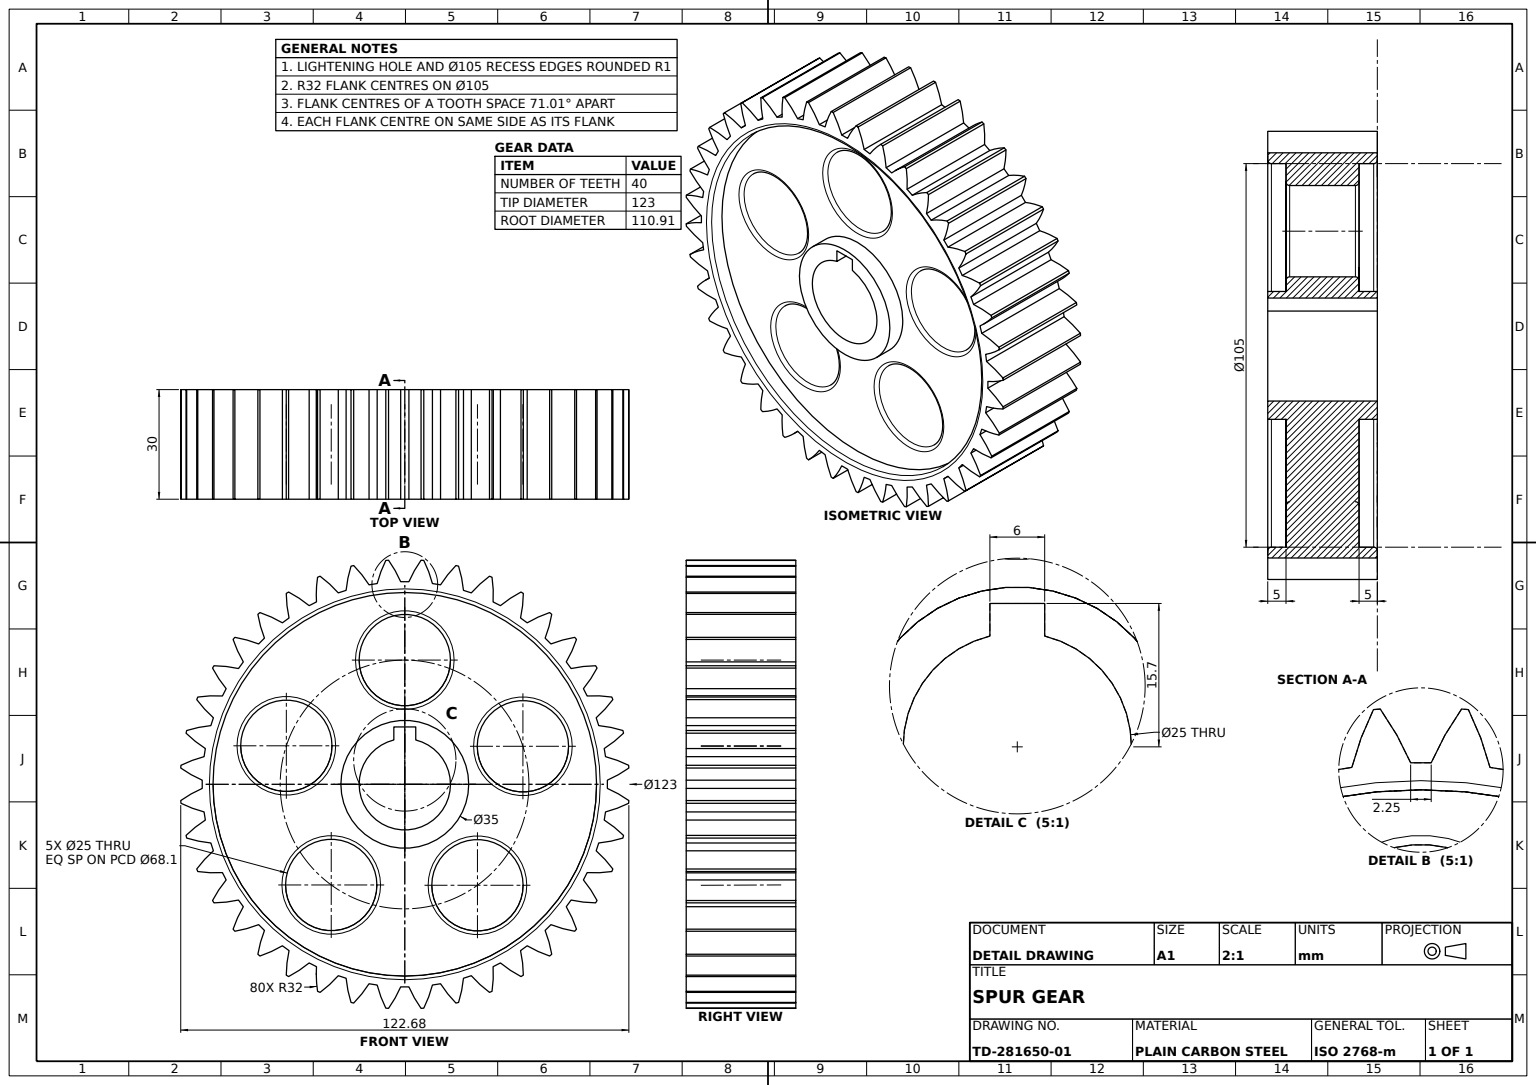
SolidWorks part; units mm, degrees
material "Plain Carbon Steel"
ref_plane "Front Plane" through (0, 0, 0) normal (0, 0, 1) x (1, 0, 0)
ref_plane "Top Plane" through (0, 0, 0) normal (0, 1, 0) x (1, 0, 0)
ref_plane "Right Plane" through (0, 0, 0) normal (1, 0, 0) x (0, 0, -1)
sketch "Gear Blank Sketch" plane through (0, 0, 0) normal (0, 0, 1) x (1, 0, 0)
  line L0 (-71.0252, 0) -> (67.6964, 0) construction
  line L1 (0, 44.8674) -> (0, -38.0607) construction
  line L2 (-3, 12.1347) -> (-3, 15.7)
  line L3 (3, 12.1347) -> (3, 15.7)
  line L4 (-3, 15.7) -> (3, 15.7)
  arc A0 (-3, 12.1347) -> (3, 12.1347) centre (0, 0) ccw
  circle A1 centre (0, 0) radius 61.5
  dimension "D1" = 25
  dimension "D4" = 123
  dimension "D2" = 6
  dimension "D3" = 15.7
extrude "Gear Blank" add sketch "Gear Blank Sketch" along normal blind 30
sketch "Face Recess Sketch" plane through (0, 0, 30) normal (0, 0, 1) x (1, 0, 0)
  circle A0 centre (0, 0) radius 52.5
  dimension "D1" = 105
extrude "Face Recess Ø105" cut sketch "Face Recess Sketch" against normal blind 5
ref_plane "Gear Mid Plane" through (0, 0, 15) normal (0, 0, 1) x (1, 0, 0)
mirror "Face Recess Mirror" about plane through (0, 0, 15) normal (0, 0, 1) of "Face Recess Ø105"
sketch "Tooth Space Sketch" plane through (0, 0, 25) normal (0, 0, 1) x (1, 0, 0)
  line L1 (0, 82.4606) -> (0, -88.1983) construction
  line L2 (-105.0435, 0) -> (137.9983, 0) construction
  line L3 (-1.125, 55.4564) -> (1.125, 55.4564)
  circle A3 centre (0, 0) radius 52.5 construction
  arc A6 (-1.125, 55.4564) -> (-4.45, 61.3388) centre (-30.4895, 42.7392) ccw
  arc A7 (1.125, 55.4564) -> (4.45, 61.3388) centre (30.4895, 42.7392) cw
  arc A10 (4.45, 61.3388) -> (-4.45, 61.3388) centre (0, 0) ccw
  dimension "D3" = 32
  dimension "D1" = 61.5
  dimension "D2" = 4.45
  dimension "D4" = 2.25
extrude "Tooth Space Cut" cut sketch "Tooth Space Sketch" against normal through all both and the other way through all
pattern_circular "Tooth Space Pattern 40x" count 40 over 360 about axis through (0, 0, 0) along (0, 0, 1) of "Tooth Space Cut"
sketch "Hub Boss Sketch" plane through (0, 0, 25) normal (0, 0, 1) x (1, 0, 0)
  line L0 (3, 15.7) -> (-3, 15.7) construction
  line L1 (3, 12.1347) -> (3, 15.7) construction
  line L2 (-3, 15.7) -> (-3, 12.1347) construction
  line L3 (3, 15.7) -> (-3, 15.7)
  line L4 (3, 12.1347) -> (3, 15.7)
  line L5 (-3, 15.7) -> (-3, 12.1347)
  arc A0 (-3, 12.1347) -> (3, 12.1347) centre (0, 0) ccw construction
  arc A3 (-3, 12.1347) -> (3, 12.1347) centre (0, 0) ccw
  circle A4 centre (0, 0) radius 17.5
  dimension "D2" = 35
extrude "Hub Boss Ø35" add sketch "Hub Boss Sketch" along normal blind 5
mirror "Hub Boss Mirror" about plane through (0, 0, 15) normal (0, 0, 1) of "Hub Boss Ø35"
sketch "Lightening Holes Sketch" plane through (0, 0, 25) normal (0, 0, 1) x (1, 0, 0)
  line L0 (0, 122.2353) -> (0, -122.6579) construction
  line L1 (-179.8138, 0) -> (206.8598, 0) construction
  circle A0 centre (0, 0) radius 52.5 construction
  circle A2 centre (0, 34) radius 12.5
  circle A3 centre (32.431, 10.5375) radius 12.5
  circle A4 centre (20.1386, -27.5566) radius 12.5
  circle A5 centre (-19.8896, -27.6375) radius 12.5
  circle A6 centre (-32.3359, 10.4066) radius 12.5
  point P17 (0.0688, -0.05)
  dimension "D1" = 25
  dimension "D2" = 34
  dimension "D4" = 0.0688
  dimension "D5" = 20.1386
  dimension "D3" = 5
extrude "Lightening Holes" cut sketch "Lightening Holes Sketch" against normal through all both and the other way through all
fillet "Edge Fillets R1" radius 1 12 edges at (32.6386, -27.5566, 25) (-7.3896, -27.6375, 25) (44.931, 10.5375, 25) (-19.8359, 10.4066, 25) (12.5, 34, 25) (-32.3896, -27.6375, 5) (7.6386, -27.5566, 5) (19.931, 10.5375, 5) (-44.8359, 10.4066, 5) (-12.5, 34, 5) (52.5, 0, 0) (52.5, 0, 30)
